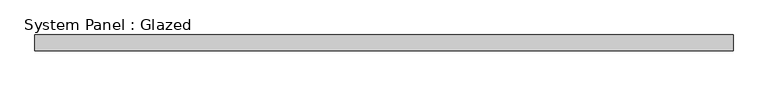
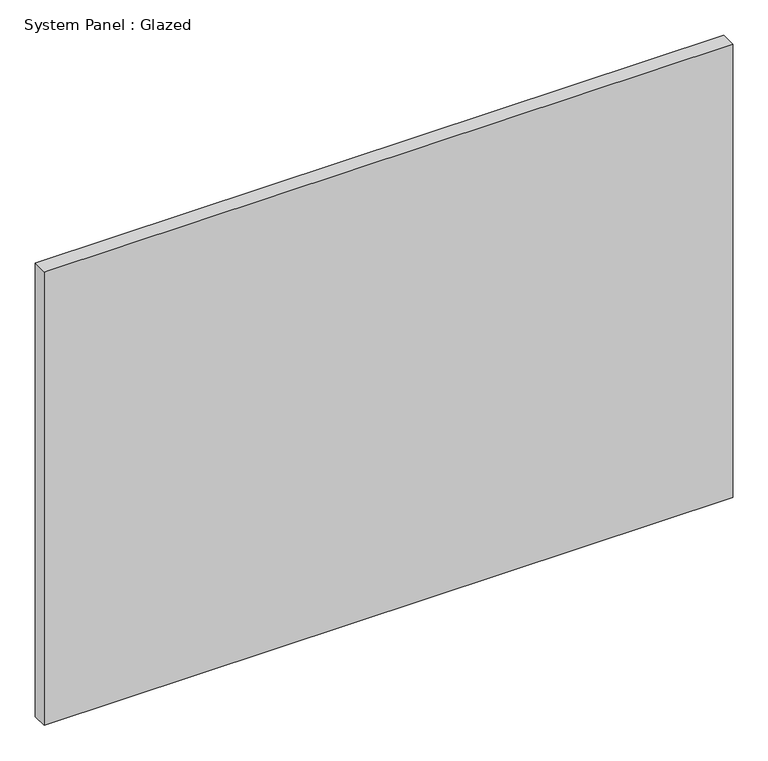
"""IFC4 building model written with IfcOpenShell, lengths in millimetres: plate geometry, System Panel : Glazed."""

from ifc_helpers import new_model, si_unit, origin, origin_with_axes, place, context, project, spatial, polyline, outline, extrude, source, transform, mapped, element, save


def system_panel_glazed_47051e8e(model_context):
    return source(origin(), model_context, "Body", "SweptSolid", [
        extrude(outline(polyline([(565.15, 19.05), (-565.15, 19.05), (-565.15, 44.45), (565.15, 44.45), (565.15, 19.05)])), origin_with_axes(), (0.0, 0.0, 1.0), 787.4),
    ])


if __name__ == "__main__":
    model = new_model("IFC4")
    model_context = context("Model", 3, world=origin())
    ifc_project = project(units=[si_unit("LENGTHUNIT", "METRE", prefix="MILLI")], contexts=[model_context])
    site = spatial("IfcSite", under=ifc_project)
    building = spatial("IfcBuilding", under=site)
    placement = place(None, origin())
    system_panel_glazed_shape = system_panel_glazed_47051e8e(model_context)
    element("IfcPlate", 1, ObjectType="System Panel : Glazed", at=placement, inside=building, context=model_context, shape_type="MappedRepresentation", body=[
        mapped(system_panel_glazed_shape, transform((0.0, 0.0, 0.0), x_axis=(1.0, 0.0, 0.0), y_axis=(0.0, 1.0, 0.0), z_axis=(0.0, 0.0, 1.0))),
    ])
    save(model, "model.ifc")

# Revit data of these elements
# Type "System Panel : Glazed"
#   Construction Type Id = "GSP4R"
#   Analytic Construction = "1/8 in Pilkington single glazing"
#   Visual Light Transmittance = 0.9
#   Solar Heat Gain Coefficient = 0.86
#   Heat Transfer Coefficient (U) = 1.18115 BTU/(h·ft²·°F)
# Element 1 (IfcPlate, "System Panel : Glazed")
#   Materials on its faces: "Glass"
# Materials
#   "Glass": class "Glass", colour RGB 0 128 192, transparency 0.75, Description = "Soda Lime Glass", Cost = 0
